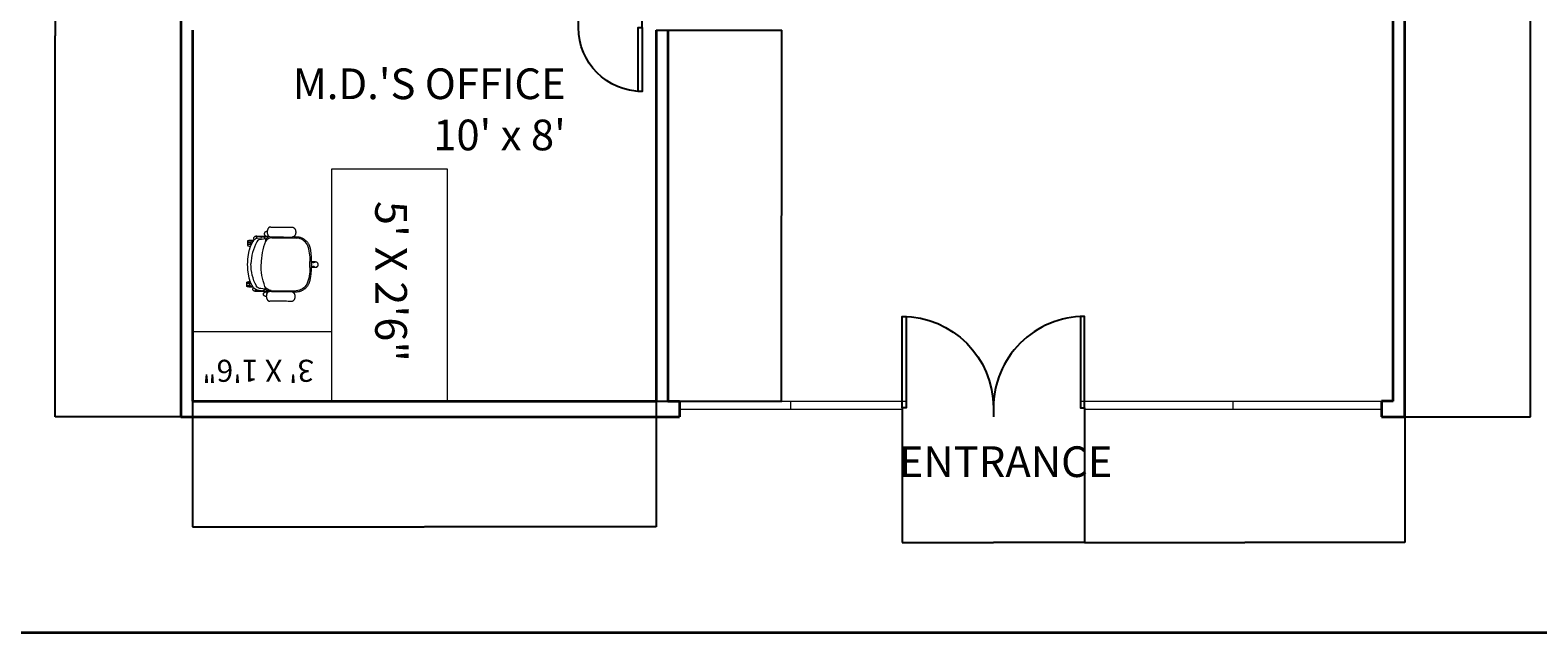
# Model space of a CAD drawing. Units: millimetres. Extents: x -5297 to 19051, y -14478 to 4427.
# Tile 1 of 4: x 1131 to 10888, y -14478 to -10580. Entities that reach past the tile are written whole.
import ezdxf

# ---------------------------------------------------------------- set-up
doc = ezdxf.new("R2010")
doc.units = ezdxf.units.MM
for name, color, linetype, lineweight in [('A-ANNO-DIMS', 2, 'Continuous', 18), ('A-ANNO-TEXT', 7, 'Continuous', 18), ('A-ANNO-TTLB', 7, 'Continuous', 35), ('A-AREA-IDEN', 7, 'Continuous', 25), ('A-DOOR', 3, 'Continuous', 25), ('A-FURN', 8, 'Continuous', 18), ('A-GLAZ', 4, 'Continuous', 18), ('A-WALL', 7, 'Continuous', 35)]:
    doc.layers.add(name, color=color, linetype=linetype, lineweight=lineweight)
doc.styles.get("Standard").update_dxf_attribs({"font": 'arial.ttf'})
doc.dimstyles.get("Standard").update_dxf_attribs({"dimtxt": 0.18, "dimasz": 0.18, "dimexe": 0.18, "dimexo": 0.0625, "dimgap": 0.09, "dimtad": 0, "dimtih": 1, "dimtoh": 1, "dimdec": 4, "dimzin": 0, "dimdsep": 46, "dimtxsty": 'Standard', "dimcen": 0.09, "dimadec": 0, "dimazin": 0, "dimtfac": 1, "dimtdec": 4, "dimtofl": 0, "dimtmove": 0, "dimatfit": 3, "dimfxl": 1, "dimtolj": 1, "dimtzin": 0, "dimarcsym": 0})

# ---------------------------------------------------------------- blocks, each defined once
blk = doc.blocks.new('*U2')
for p, q in [((-700, 0), (-700, -100)), ((0, 0), (0, -100))]:
    blk.add_line(p, q)
blk.add_lwpolyline([(0, 0), (0, 700), (-43.75, 700), (-43.75, 0)], close=True)
blk.add_arc((0, 0), 700, 90, 180)
blk = doc.blocks.new('fdss')
at = {"color": 0}
for p, q in [((426, 240), (196, 239)), ((470, 236), (480, 226)), ((480, 225), (479, 223)), ((482, 204), (480, 210)), ((484, 228), (520, 224)), ((617, 196), (646, 196)), ((618, 179), (646, 179)), ((647, 195), (647, 179)), ((426, -240), (196, -239)), ((470, -236), (480, -226)), ((480, -225), (479, -223)), ((482, -204), (480, -210)), ((484, -228), (520, -224)), ((617, -196), (646, -196)), ((618, -179), (646, -179)), ((647, -195), (647, -179))]:
    blk.add_line(p, q, dxfattribs=at)
for points in [[(505, 245), (520, 247), (546, 249), (551, 249)], [(566, 236), (554, 235), (512, 240)], [(33, 21), (34, 20), (36, 19), (37, 18), (37, 18), (39, 18)], [(39, 18), (41, 17), (43, 17), (46, 16), (47, 16), (50, 16), (53, 16), (55, 16), (57, 16), (60, 16), (63, 16)], [(75, -28), (75, 0), (75, 28)], [(33, -21), (34, -20), (36, -19), (37, -18), (37, -18), (39, -18)], [(39, -18), (41, -17), (43, -17), (46, -16), (47, -16), (50, -16), (53, -16), (55, -16), (57, -16), (60, -16), (63, -16)], [(505, -245), (520, -247), (546, -249), (551, -249)], [(566, -236), (554, -235), (512, -240)]]:
    blk.add_lwpolyline(points, dxfattribs=at)
at = {"color": 0, "extrusion": (0, 0, -1)}
for centre, major_axis, start_param, end_param in [((445, 42), (-262, 262), 5.459154, 5.874691), ((201, 128), (-79, 79), 5.969012, 7.027382), ((424, 173), (47, 47), -0.751727, 0.301996), ((424, 175), (54.1, 54.1), -0.544214, -0.156468), ((514, 220), (24.9, 24.9), 3.662908, 4.015109), ((484, 224), (3.3, 3.3), 4.243712, 5.205719), ((484, 229), (-1.47, 1.47), 3.927418, 5.578652), ((-41, 3), (553, 91), -0.204201, 0.167634), ((500, 224), (-12.9, 12.9), 5.819354, 6.506047), ((509, 207), (26.9, 26.9), -1.329065, -0.883773), ((521, 177), (-33.1, 33.1), 0.763307, 1.830683), ((550, 228), (14.8, 14.8), -0.735707, 0.161366), ((545, 180), (-39.3, 39.3), 0.935679, 1.762262), ((193, 0), (-296, 296), 1.856147, 2.355859), ((566, 238), (1.31, 1.31), 0.929037, 2.293349), ((563, 238), (-2.9, 2.9), 1.793197, 2.458506), ((597, 186), (15.6, 15.6), -0.947253, 1.474381), ((621, 198), (-1.12, 1.12), 2.396655, 3.926991), ((621, 177), (-1.12, 1.12), 0.785398, 2.315734), ((646, 195), (0.539, 0.539), -0.785398, 0.785398), ((646, 179), (-0.539, 0.539), 2.356195, 3.926991)]:
    blk.add_ellipse(centre, major_axis=major_axis, ratio=1, start_param=start_param, end_param=end_param, dxfattribs=at)
at = {"color": 0}
for centre, major_axis, start_param, end_param in [((445, -42), (262, 262), 2.317561, 2.733098), ((-41, -3), (-553, 91), 2.937392, 3.309227), ((193, 0), (296, 296), 4.99774, 5.497452), ((201, -128), (79, 79), 2.82742, 3.885789), ((424, -173), (-47, 47), 2.389866, 3.443588), ((424, -175), (-54.1, 54.1), 2.597378, 2.985125), ((514, -220), (-24.9, 24.9), 0.521315, 0.873517), ((484, -224), (-3.3, 3.3), 1.102119, 2.064126), ((484, -229), (1.47, 1.47), 0.785825, 2.437059), ((500, -224), (12.9, 12.9), 2.677762, 3.364454), ((509, -207), (-26.9, 26.9), 1.812527, 2.25782), ((521, -177), (33.1, 33.1), 3.9049, 4.972275), ((550, -228), (-14.8, 14.8), 2.405886, 3.302959), ((545, -180), (39.3, 39.3), 4.077272, 4.903855), ((566, -238), (-1.31, 1.31), 4.07063, 5.434941), ((563, -238), (2.9, 2.9), 4.93479, 5.600098), ((597, -186), (15.6, 15.6), 3.765136, 6.18677), ((621, -177), (1.12, 1.12), 3.926991, 5.457327), ((621, -198), (1.12, 1.12), 5.538248, 7.068583), ((646, -179), (0.539, 0.539), 5.497787, 7.068583), ((646, -195), (-0.539, 0.539), 2.356195, 3.926991)]:
    blk.add_ellipse(centre, major_axis=major_axis, ratio=1, start_param=start_param, end_param=end_param, dxfattribs=at)
for points, weights, knots in [([(436, 337), (338, 337), (240, 337), (234, 338), (228, 335), (217, 328), (212, 315), (204, 293), (212, 271), (217, 258), (228, 251), (234, 248), (240, 248)], [1, 1, 1, 0.962754439438, 1, 0.939418827348, 1, 0.934055427035, 1, 0.939418827348, 1, 0.962754439438, 1], [0, 0, 0, 1, 1, 1.54757, 1.54757, 2.247301, 2.247301, 2.977684, 2.977684, 3.677415, 3.677415, 4.224984, 4.224984, 4.224984]), ([(436, 337), (443, 338), (449, 335), (460, 328), (464, 315), (473, 293), (464, 271), (460, 258), (449, 251), (443, 248), (436, 248), (338, 248), (240, 248)], [1, 0.96275443944, 1, 0.939418827348, 1, 0.934055427035, 1, 0.939418827348, 1, 0.96275443944, 1, 1, 1], [0, 0, 0, 0.54757, 0.54757, 1.247301, 1.247301, 1.977684, 1.977684, 2.677415, 2.677415, 3.224984, 3.224984, 4.224984, 4.224984, 4.224984]), ([(468, 296), (480, 296), (489, 288), (493, 285), (494, 280), (496, 274), (494, 268), (488, 255), (474, 254), (463, 254), (452, 253)], [1, 0.943338632687, 1, 0.968267368414, 1, 0.9394851057, 1, 0.864198855487, 1, 1, 1], [0, 0, 0, 0.676489, 0.676489, 1.181677, 1.181677, 1.881021, 1.881021, 2.935502, 2.935502, 3.935502, 3.935502, 3.935502]), ([(227, 252), (219, 252), (211, 252), (156, 255), (115, 218), (74, 180), (72, 125), (63, 75), (63, 25), (63, 13), (62, 0), (63, -13), (63, -25), (63, -75), (72, -125), (74, -180), (115, -218), (156, -255), (211, -252), (219, -252), (227, -252)], [1, 1, 1, 0.920970329426, 1, 0.920970329426, 1, 0.996764637726, 1, 1, 1, 1, 1, 0.996764637726, 1, 0.920970329426, 1, 0.920970329426, 1, 1, 1], [0, 0, 0, 1, 1, 1.800466, 1.800466, 2.600931, 2.600931, 2.761856, 2.761856, 3.761856, 3.761856, 4.761856, 4.761856, 4.922781, 4.922781, 5.723247, 5.723247, 6.523712, 6.523712, 7.523712, 7.523712, 7.523712]), ([(447, 248), (506, 249), (566, 251), (577, 251), (585, 244), (591, 239), (592, 232), (592, 228), (590, 225), (589, 221), (585, 219)], [1, 1, 1, 0.935512434708, 1, 0.918468104225, 1, 0.965843473499, 1, 0.972653000165, 1], [0, 0, 0, 1, 1, 1.722179, 1.722179, 2.535393, 2.535393, 3.059628, 3.059628, 3.528435, 3.528435, 3.528435]), ([(591, 211), (619, 173), (629, 128), (645, 65), (645, 0), (645, -65), (629, -128), (619, -173), (591, -211)], [1, 0.979760898136, 1, 0.992391068779, 1, 0.992391068779, 1, 0.979760898136, 1], [0, 0, 0, 0.403066, 0.403066, 0.649944, 0.649944, 0.896822, 0.896822, 1.299888, 1.299888, 1.299888]), ([(592, 211), (618, 216), (643, 209), (646, 209), (646, 206), (646, 203), (646, 199), (646, 198), (644, 198), (630, 198), (616, 198)], [1, 0.974666881773, 1, 0.783317345499, 1, 1, 1, 0.707106807826, 1, 1, 1], [0, 0, 0, 0.451139, 0.451139, 1.792762, 1.792762, 2.792762, 2.792762, 4.363559, 4.363559, 5.363559, 5.363559, 5.363559]), ([(618, 177), (631, 177), (644, 177), (645, 177), (645, 176), (646, 176), (646, 175), (646, 172), (646, 168), (646, 166), (643, 165), (631, 161), (619, 161)], [1, 1, 1, 0.923879528314, 1, 0.923879528314, 1, 1, 1, 0.783317456604, 1, 0.992237440768, 1], [0, 0, 0, 1, 1, 1.785398, 1.785398, 2.570796, 2.570796, 3.570796, 3.570796, 4.912419, 4.912419, 5.161781, 5.161781, 5.161781]), ([(33, -20), (22, -27), (10, -20), (-1, -13), (0, 0), (-1, 13), (10, 20), (22, 27), (33, 20)], [1, 0.85579821339, 1, 0.85579821339, 1, 0.855798213391, 1, 0.855798213391, 1], [0, 0, 0, 1.087409, 1.087409, 2.174818, 2.174818, 3.262227, 3.262227, 4.349636, 4.349636, 4.349636]), ([(12, 21), (13, 23), (15, 23), (39, 29), (63, 25)], [1, 0.873023611703, 1, 0.980536821249, 1], [0, 0, 0, 1.018856, 1.018856, 1.414094, 1.414094, 1.414094]), ([(12, -21), (13, -23), (15, -23), (39, -29), (63, -25)], [1, 0.873023611717, 1, 0.980536821249, 1], [0, 0, 0, 1.018856, 1.018856, 1.414094, 1.414094, 1.414094]), ([(464, -271), (460, -258), (449, -251), (443, -248), (436, -248), (338, -248), (240, -248), (234, -248), (228, -251), (217, -258), (212, -271), (204, -293), (212, -315), (217, -328), (228, -335), (234, -338), (240, -337), (338, -337), (436, -337)], [1, 0.939418827349, 1, 0.96275443944, 1, 1, 1, 0.962754439438, 1, 0.939418827349, 1, 0.934055427035, 1, 0.939418827348, 1, 0.962754439438, 1, 1, 1], [0, 0, 0, 0.699731, 0.699731, 1.247301, 1.247301, 2.247301, 2.247301, 2.794871, 2.794871, 3.494602, 3.494602, 4.224984, 4.224984, 4.924715, 4.924715, 5.472285, 5.472285, 6.472285, 6.472285, 6.472285]), ([(464, -271), (473, -293), (464, -315), (460, -328), (449, -335), (443, -338), (436, -337)], [1, 0.934055427035, 1, 0.939418827348, 1, 0.96275443944, 1], [0, 0, 0, 0.730383, 0.730383, 1.430114, 1.430114, 1.977684, 1.977684, 1.977684]), ([(447, -248), (506, -249), (566, -251), (577, -251), (585, -244), (591, -239), (592, -232), (592, -228), (590, -225), (589, -221), (585, -219)], [1, 1, 1, 0.935512434708, 1, 0.918468104224, 1, 0.965843473499, 1, 0.972653000166, 1], [0, 0, 0, 1, 1, 1.722179, 1.722179, 2.535393, 2.535393, 3.059628, 3.059628, 3.528435, 3.528435, 3.528435]), ([(468, -296), (480, -296), (489, -288), (493, -285), (494, -280), (496, -274), (494, -268), (488, -255), (474, -254), (463, -254), (452, -253)], [1, 0.943338632687, 1, 0.968267368413, 1, 0.9394851057, 1, 0.864198855486, 1, 1, 1], [0, 0, 0, 0.676489, 0.676489, 1.181677, 1.181677, 1.881021, 1.881021, 2.935502, 2.935502, 3.935502, 3.935502, 3.935502]), ([(592, -211), (618, -216), (643, -209), (646, -209), (646, -206), (646, -203), (646, -199), (646, -198), (644, -198), (630, -198), (616, -198)], [1, 0.974666881774, 1, 0.7833173455, 1, 1, 1, 0.707106807832, 1, 1, 1], [0, 0, 0, 0.451139, 0.451139, 1.792762, 1.792762, 2.792762, 2.792762, 4.363559, 4.363559, 5.363559, 5.363559, 5.363559]), ([(618, -177), (631, -177), (644, -177), (645, -177), (645, -176), (646, -176), (646, -175), (646, -172), (646, -168), (646, -166), (643, -165), (631, -161), (619, -161)], [1, 1, 1, 0.923879528318, 1, 0.923879528318, 1, 1, 1, 0.783317456602, 1, 0.992237440768, 1], [0, 0, 0, 1, 1, 1.785398, 1.785398, 2.570796, 2.570796, 3.570796, 3.570796, 4.912419, 4.912419, 5.161781, 5.161781, 5.161781])]:
    blk.add_rational_spline(points, weights, degree=2, knots=knots, dxfattribs=at)
blk = doc.blocks.new('*U8')
for p, q in [((0, 0), (0, 100)), ((1000, 0), (1000, 100))]:
    blk.add_line(p, q)
blk.add_lwpolyline([(0, 0), (0, -1000), (43.75, -1000), (43.75, 0)], close=True)
blk.add_arc((0, 0), 1000, 270, 0)
blk = doc.blocks.new('*D21')
at = {"layer": 'A-ANNO-DIMS', "color": 0, "lineweight": -2, "transparency": 16777216}
for p, q in [((10028, 2246.2), (10840.6, 2246.2)), ((10840.4, 2246), (10840.4, -5417.6)), ((10840.4, -13081.5), (10840.4, -5417.9)), ((10028, -13081.7), (10840.6, -13081.7))]:
    blk.add_line(p, q, dxfattribs=at)
at = {"layer": 'A-ANNO-DIMS', "color": 0, "transparency": 16777216}
for points in [[(10840.4, 2246), (10840.4, 2246), (10840.4, 2246.2)], [(10840.4, -13081.5), (10840.4, -13081.5), (10840.4, -13081.7)]]:
    blk.add_solid(points, dxfattribs=at)
at = {"layer": 'Defpoints', "color": 0, "transparency": 16777216}
for p in [(10027.9, 2246.2), (10027.9, -13081.7), (10840.4, -13081.7)]:
    blk.add_point(p, dxfattribs=at)
at = {"layer": 'A-ANNO-DIMS', "color": 0, "transparency": 16777216, "insert": (10840.4, -5417.8), "char_height": 0.18, "attachment_point": 5}
blk.add_mtext('\\A1;15328', dxfattribs=at)
blk = doc.blocks.new('*D22')
at = {"layer": 'A-ANNO-DIMS', "color": 0, "lineweight": -2, "transparency": 16777216}
for p, q in [((2105.4, -8153), (1292.8, -8153)), ((1293, -8153.2), (1293, -10616.8)), ((1293, -13080.7), (1293, -10617.1)), ((2105.4, -13080.9), (1292.8, -13080.9))]:
    blk.add_line(p, q, dxfattribs=at)
at = {"layer": 'A-ANNO-DIMS', "color": 0, "transparency": 16777216}
for points in [[(1293, -8153.2), (1293, -8153.2), (1293, -8153)], [(1293, -13080.7), (1293, -13080.7), (1293, -13080.9)]]:
    blk.add_solid(points, dxfattribs=at)
at = {"layer": 'Defpoints', "color": 0, "transparency": 16777216}
for p in [(1293, -8153), (2105.5, -8153), (2105.5, -13080.9)]:
    blk.add_point(p, dxfattribs=at)
at = {"layer": 'A-ANNO-DIMS', "color": 0, "transparency": 16777216, "insert": (1293, -10617), "char_height": 0.18, "attachment_point": 5}
blk.add_mtext('\\A1;4928', dxfattribs=at)
blk = doc.blocks.new('*D25')
at = {"layer": 'A-ANNO-DIMS', "color": 0, "lineweight": -2, "transparency": 16777216}
for p, q in [((7955, -13081.4), (7954.8, -13894)), ((10027.9, -13081.8), (10027.8, -13894.4)), ((7955, -13893.9), (8990.9, -13894)), ((10027.6, -13894.2), (8991.7, -13894))]:
    blk.add_line(p, q, dxfattribs=at)
at = {"layer": 'A-ANNO-DIMS', "color": 0, "transparency": 16777216}
for points in [[(7955, -13893.8), (7955, -13893.9), (7954.8, -13893.9)], [(10027.6, -13894.2), (10027.6, -13894.2), (10027.8, -13894.2)]]:
    blk.add_solid(points, dxfattribs=at)
at = {"layer": 'Defpoints', "color": 0, "transparency": 16777216}
for p in [(7955, -13081.4), (10027.9, -13081.7), (7954.8, -13893.9)]:
    blk.add_point(p, dxfattribs=at)
at = {"layer": 'A-ANNO-DIMS', "color": 0, "transparency": 16777216, "insert": (8991.3, -13894), "char_height": 0.18, "attachment_point": 5}
blk.add_mtext('\\A1;2073', dxfattribs=at)
blk = doc.blocks.new('*D26')
at = {"layer": 'A-ANNO-DIMS', "color": 0, "lineweight": -2, "transparency": 16777216}
for p, q in [((6773.9, -13081.4), (6773.9, -13894)), ((7955, -13081.4), (7955, -13894)), ((6774.1, -13893.9), (7364.1, -13893.9)), ((7954.8, -13893.9), (7364.8, -13893.9))]:
    blk.add_line(p, q, dxfattribs=at)
at = {"layer": 'A-ANNO-DIMS', "color": 0, "transparency": 16777216}
for points in [[(6774.1, -13893.8), (6774.1, -13893.9), (6773.9, -13893.9)], [(7954.8, -13893.8), (7954.8, -13893.9), (7955, -13893.9)]]:
    blk.add_solid(points, dxfattribs=at)
at = {"layer": 'Defpoints', "color": 0, "transparency": 16777216}
for p in [(6773.9, -13081.4), (7955, -13081.4), (6773.9, -13893.9)]:
    blk.add_point(p, dxfattribs=at)
at = {"layer": 'A-ANNO-DIMS', "color": 0, "transparency": 16777216, "insert": (7364.4, -13893.9), "char_height": 0.18, "attachment_point": 5}
blk.add_mtext('\\A1;1181', dxfattribs=at)
blk = doc.blocks.new('*D39')
at = {"layer": 'A-ANNO-DIMS', "color": 0, "lineweight": -2, "transparency": 16777216}
for p, q in [((2181.7, -12980.1), (2181.7, -13792.7)), ((5181.7, -12980.1), (5181.7, -13792.7)), ((2181.9, -13792.5), (3681.3, -13792.5)), ((5181.5, -13792.5), (3682.1, -13792.5))]:
    blk.add_line(p, q, dxfattribs=at)
at = {"layer": 'A-ANNO-DIMS', "color": 0, "transparency": 16777216}
for points in [[(2181.9, -13792.5), (2181.9, -13792.5), (2181.7, -13792.5)], [(5181.5, -13792.5), (5181.5, -13792.5), (5181.7, -13792.5)]]:
    blk.add_solid(points, dxfattribs=at)
at = {"layer": 'Defpoints', "color": 0, "transparency": 16777216}
for p in [(2181.7, -12980), (5181.7, -12980), (2181.7, -13792.5)]:
    blk.add_point(p, dxfattribs=at)
at = {"layer": 'A-ANNO-DIMS', "color": 0, "transparency": 16777216, "insert": (3681.7, -13792.5), "char_height": 0.18, "attachment_point": 5}
blk.add_mtext('\\A1;3000', dxfattribs=at)
blk = doc.blocks.new('*D40')
at = {"layer": 'A-ANNO-DIMS', "color": 0, "lineweight": -2, "transparency": 16777216}
for p, q in [((5181.8, -10580), (5994.4, -10580)), ((5994.2, -10580.2), (5994.2, -11779.8)), ((5994.2, -12979.8), (5994.2, -11780.2)), ((5181.8, -12980), (5994.4, -12980))]:
    blk.add_line(p, q, dxfattribs=at)
at = {"layer": 'A-ANNO-DIMS', "color": 0, "transparency": 16777216}
for points in [[(5994.2, -10580.2), (5994.2, -10580.2), (5994.2, -10580)], [(5994.2, -12979.8), (5994.2, -12979.8), (5994.2, -12980)]]:
    blk.add_solid(points, dxfattribs=at)
at = {"layer": 'Defpoints', "color": 0, "transparency": 16777216}
for p in [(5181.7, -10580), (5181.7, -12980), (5994.2, -12980)]:
    blk.add_point(p, dxfattribs=at)
at = {"layer": 'A-ANNO-DIMS', "color": 0, "transparency": 16777216, "insert": (5994.2, -11780), "char_height": 0.18, "attachment_point": 5}
blk.add_mtext('\\A1;2400', dxfattribs=at)

msp = doc.modelspace()

# ---------------------------------------------------------------- linework, layer by layer
at = {"layer": 'A-ANNO-TTLB'}
msp.add_lwpolyline([(-5297.04, 4427.15), (19050.7, 4427.15), (19050.7, -14478.12), (-5297.04, -14478.12)], close=True, dxfattribs=at)
at = {"layer": 'A-DOOR'}
msp.add_line((7362.92, -12980.01), (7365.95, -12980.01), dxfattribs=at)
at = {"layer": 'A-FURN'}
for p, q in [((3831.7, -11480.01), (3081.7, -11480.01)), ((3081.7, -11480.01), (3081.7, -12980.01)), ((3831.7, -12980.01), (3831.7, -11480.01)), ((2181.7, -12980.01), (2181.7, -12530.01)), ((2181.7, -12530.01), (3081.7, -12530.01)), ((3081.7, -12980.01), (2181.7, -12980.01)), ((3081.7, -12980.01), (3831.7, -12980.01))]:
    msp.add_line(p, q, dxfattribs=at)
at = {"layer": 'A-GLAZ'}
for p, q in [((5257.9, -12980.01), (6799.74, -12980.01)), ((5334.1, -13030.61), (6773.9, -13030.68)), ((6054, -13030.64), (6054, -12980.01)), ((7929.14, -12980.01), (9951.7, -12980.01)), ((7954.98, -13030.74), (9875.5, -13030.84)), ((8915.24, -13030.79), (8915.24, -12980.01))]:
    msp.add_line(p, q, dxfattribs=at)
at = {"layer": 'A-WALL'}
for p, q in [((2105.5, 2246.19), (2105.5, -13080.86)), ((10027.9, -13081.69), (10027.9, 2246.19)), ((9951.7, -12980.01), (9951.7, -6303.81)), ((2181.7, -10580.01), (2181.7, -12980.01)), ((5181.7, -10580.01), (5181.7, -12980.01)), ((5257.9, -10580.01), (5257.9, -12980.01)), ((2181.7, -12980.01), (5181.7, -12980.01)), ((5257.9, -12980.01), (5334.1, -12980.01)), ((5334.1, -12980.01), (5334.09, -13081.2)), ((9875.5, -12980.01), (9875.49, -13081.68)), ((9951.7, -12980.01), (9875.5, -12980.01)), ((2105.5, -13080.86), (5334.09, -13081.2)), ((9875.49, -13081.68), (10027.9, -13081.69))]:
    msp.add_line(p, q, dxfattribs=at)

# ---------------------------------------------------------------- block references
at = {"layer": 'A-DOOR', "yscale": 0.5905371076916341, "zscale": 0.5905371076916341, "rotation": 180}
for name, p, xscale in [('*U2', (5092.22, -10562.86), -0.5905371076916341), ('*U8', (6773.9, -13022.3), -0.5905371076916341), ('*U8', (7954.98, -13022.3), 0.5905371076916341)]:
    msp.add_blockref(name, p, dxfattribs=dict(at, xscale=xscale))
at = {"layer": 'A-FURN', "xscale": -0.7108527329127514, "yscale": 0.7108527329127514, "zscale": 0.7108527329127514, "rotation": 359.2672508438734}
msp.add_blockref('fdss', (2994.79, -12096.9), dxfattribs=at)

# ---------------------------------------------------------------- texts
at = {"layer": 'A-ANNO-TEXT'}
for s, width, gutter_width, insert, char_height, attachment_point, rotation in [('{\\fArial|b1|i0|c0|p34;5\' X 2\'6"}', 2729.7181, 427.84, (3363.87, -11684.41), 205.365, 7, 270), ('{\\fArial|b1|i0|c0|p34;3\' X 1\'6"}', 1895.1096, 297.03, (2245.01, -12854.37), 142.5749, 3, 180)]:
    msp.add_mtext_dynamic_manual_height_columns(s, width=width, gutter_width=gutter_width, heights=[0], dxfattribs=dict(at, insert=insert, char_height=char_height, attachment_point=attachment_point, rotation=rotation))
at = {"layer": 'A-AREA-IDEN', "char_height": 198.615, "attachment_point": 3}
for s, width, insert in [("{\\fArial|b1|i0|c0|p34;M.D.'S OFFICE ^J    10' x 8'  }", 1957.0622, (4596.98, -10827.46)), ('{\\fArial|b1|i0|c0|p34;ENTRANCE}', 1554.1615, (8134.97, -13271.85))]:
    msp.add_mtext_dynamic_manual_height_columns(s, width=width, gutter_width=413.78, heights=[0], dxfattribs=dict(at, insert=insert))

# ---------------------------------------------------------------- dimensions: what is measured, and where the dimension line sits
at = {"layer": 'A-ANNO-DIMS'}
for base, p1, p2, angle, picture, middle in [((10840.4, -13081.69), (10027.9, 2246.19), (10027.9, -13081.69), 270, '*D21', (10840.4, -5417.75)), ((1293, -8153.04), (2105.5, -13080.86), (2105.5, -8153.04), 90, '*D22', (1293, -10616.95)), ((5994.2, -12980.01), (5181.7, -10580.01), (5181.7, -12980.01), 270, '*D40', (5994.2, -11780.01)), ((2181.7, -13792.51), (5181.7, -12980.01), (2181.7, -12980.01), 180, '*D39', (3681.7, -13792.51)), ((6773.9, -13893.85), (7954.98, -13081.35), (6773.9, -13081.35), 180, '*D26', (7364.44, -13893.85)), ((7954.84, -13893.85), (10027.9, -13081.69), (7954.98, -13081.35), 179.990601, '*D25', (8991.31, -13894.02))]:
    dim = msp.add_linear_dim(base=base, p1=p1, p2=p2, angle=angle, dimstyle='Standard', override={"dimdec": 0, "dimlfac": 1, "dimrnd": 0, "dimzin": 0, "dimdsep": 46, "dimlunit": 2}, dxfattribs=at)
    dim.commit()
    dim.dimension.update_dxf_attribs({"geometry": picture, "text_midpoint": middle})

doc.saveas('drawing.dxf')
